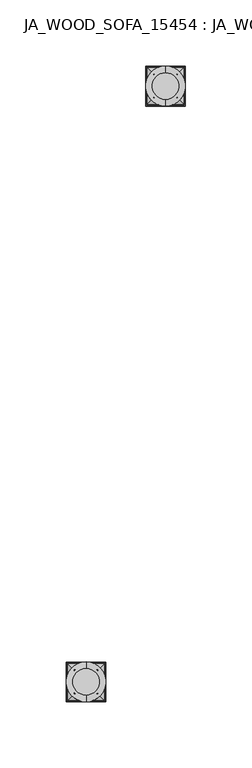
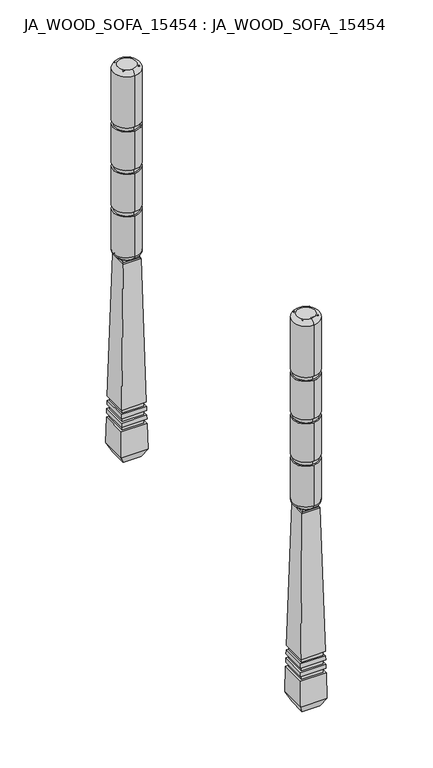
"""IFC4 building model written with IfcOpenShell, lengths in millimetres: furniture geometry, JA_WOOD_SOFA_15454 : JA_WOOD_SOFA_15454."""

from ifc_helpers import new_model, si_unit, point, frame, origin, origin_with_axes, place, context, project, spatial, polyline, circle_curve, ellipse_curve, trimmed, outline, extrude, faceted_brep, source, transform, mapped, element, save
from ifc_brep_helpers import plane_surface, cylinder_surface, revolved_surface, advanced_brep


def ja_wood_sofa_15454_ja_wood_sofa_15454_b7308ffd(model_context):
    return source(origin(), model_context, "Body", "SolidModel", [
        advanced_brep(
        [(-237.5, 460.0, 460.0), (-237.5, 440.0, 460.0), (-237.5, 442.0710678, 235.0), (-237.5, 457.9289322, 235.0), (-237.5, 465.0, 245.0), (-237.5, 465.0, 242.0710678), (-237.5, 435.0, 242.0710678), (-237.5, 435.0, 245.0), (-237.5, 435.0, 290.0), (-237.5, 465.0, 290.0), (-237.5, 465.0, 455.0000045), (-237.5, 465.0, 450.0), (-237.5, 465.0, 395.0), (-237.5, 435.0, 395.0), (-237.5, 435.0, 450.0), (-237.5, 435.0, 455.0000074), (-237.5, 465.0, 390.0), (-237.5, 465.0, 345.0), (-237.5, 435.0, 345.0), (-237.5, 435.0, 390.0), (-237.5, 465.0, 340.0), (-237.5, 465.0, 295.0), (-237.5, 435.0, 295.0), (-237.5, 435.0, 340.0), (-237.5, 436.4644661, 238.5355339), (-237.5, 463.5355339, 238.5355339), (-237.5, 461.4644661, 236.4644661), (-237.5, 438.5355339, 236.4644661), (-237.5, 437.0, 340.0), (-237.5, 437.0, 345.0), (-237.5, 463.0, 345.0), (-237.5, 463.0, 340.0), (-237.5, 437.0, 390.0), (-237.5, 437.0, 395.0), (-237.5, 463.0, 395.0), (-237.5, 463.0, 390.0), (-237.5, 437.0, 290.0), (-237.5, 437.0, 295.0), (-237.5, 463.0, 295.0), (-237.5, 463.0, 290.0)],
        [
            (0, 1, circle_curve(frame((-237.5, 450.0, 460.0), z_axis=(0.0, 0.0, 1.0), x_axis=(0.0, 1.0, 0.0)), 10.0)),
            (1, 0, circle_curve(frame((-237.5, 450.0, 460.0), z_axis=(0.0, 0.0, 1.0), x_axis=(0.0, -1.0, 0.0)), 10.0)),
            (2, 3, circle_curve(frame((-237.5, 450.0, 235.0), z_axis=(0.0, 0.0, -1.0), x_axis=(0.0, 1.0, 0.0)), 7.9289322)),
            (3, 2, circle_curve(frame((-237.5, 450.0, 235.0), z_axis=(0.0, 0.0, -1.0), x_axis=(0.0, -1.0, 0.0)), 7.9289322)),
            (4, 5),
            (5, 6, circle_curve(frame((-237.5, 450.0, 242.0710678), z_axis=(0.0, 0.0, 1.0), x_axis=(0.0, -1.0, 0.0)), 15.0)),
            (6, 7),
            (7, 8),
            (8, 9, circle_curve(frame((-237.5, 450.0, 290.0), z_axis=(0.0, 0.0, -1.0), x_axis=(0.0, -1.0, 0.0)), 15.0)),
            (9, 4),
            (10, 11),
            (11, 12),
            (12, 13, circle_curve(frame((-237.5, 450.0, 395.0), z_axis=(0.0, 0.0, 1.0), x_axis=(0.0, -1.0, 0.0)), 15.0)),
            (13, 14),
            (14, 15),
            (15, 10, circle_curve(frame((-237.5, 450.0, 455.0), z_axis=(0.0, 0.0, -1.0), x_axis=(0.0, -1.0, 0.0)), 15.0)),
            (16, 17),
            (17, 18, circle_curve(frame((-237.5, 450.0, 345.0), z_axis=(0.0, 0.0, 1.0), x_axis=(0.0, -1.0, 0.0)), 15.0)),
            (18, 19),
            (19, 16, circle_curve(frame((-237.5, 450.0, 390.0), z_axis=(0.0, 0.0, -1.0), x_axis=(0.0, -1.0, 0.0)), 15.0)),
            (20, 21),
            (21, 22, circle_curve(frame((-237.5, 450.0, 295.0), z_axis=(0.0, 0.0, 1.0), x_axis=(0.0, -1.0, 0.0)), 15.0)),
            (22, 23),
            (23, 20, circle_curve(frame((-237.5, 450.0, 340.0), z_axis=(0.0, 0.0, -1.0), x_axis=(0.0, -1.0, 0.0)), 15.0)),
            (9, 8, circle_curve(frame((-237.5, 450.0, 290.0), z_axis=(0.0, 0.0, -1.0), x_axis=(0.0, -1.0, 0.0)), 15.0)),
            (6, 5, circle_curve(frame((-237.5, 450.0, 242.0710678), z_axis=(0.0, 0.0, 1.0), x_axis=(0.0, -1.0, 0.0)), 15.0)),
            (10, 15, circle_curve(frame((-237.5, 450.0, 455.0), z_axis=(0.0, 0.0, -1.0), x_axis=(0.0, -1.0, 0.0)), 15.0)),
            (13, 12, circle_curve(frame((-237.5, 450.0, 395.0), z_axis=(0.0, 0.0, 1.0), x_axis=(0.0, -1.0, 0.0)), 15.0)),
            (16, 19, circle_curve(frame((-237.5, 450.0, 390.0), z_axis=(0.0, 0.0, -1.0), x_axis=(0.0, -1.0, 0.0)), 15.0)),
            (18, 17, circle_curve(frame((-237.5, 450.0, 345.0), z_axis=(0.0, 0.0, 1.0), x_axis=(0.0, -1.0, 0.0)), 15.0)),
            (20, 23, circle_curve(frame((-237.5, 450.0, 340.0), z_axis=(0.0, 0.0, -1.0), x_axis=(0.0, -1.0, 0.0)), 15.0)),
            (22, 21, circle_curve(frame((-237.5, 450.0, 295.0), z_axis=(0.0, 0.0, 1.0), x_axis=(0.0, -1.0, 0.0)), 15.0)),
            (24, 6, circle_curve(frame((-237.5, 440.0, 242.0710678), z_axis=(-1.0, 0.0, 0.0), x_axis=(0.0, -1.0, 0.0)), 5.0)),
            (5, 25, circle_curve(frame((-237.5, 460.0, 242.0710678), z_axis=(-1.0, 0.0, 0.0), x_axis=(0.0, 1.0, 0.0)), 5.0)),
            (25, 24, circle_curve(frame((-237.5, 450.0, 238.5355339), z_axis=(0.0, 0.0, 1.0), x_axis=(0.0, 1.0, 0.0)), 13.5355339)),
            (25, 26),
            (26, 27, circle_curve(frame((-237.5, 450.0, 236.4644661), z_axis=(0.0, 0.0, 1.0), x_axis=(0.0, 1.0, 0.0)), 11.4644661)),
            (27, 24),
            (26, 3, circle_curve(frame((-237.5, 457.9289322, 240.0), z_axis=(-1.0, 0.0, 0.0), x_axis=(0.0, 1.0, 0.0)), 5.0)),
            (2, 27, circle_curve(frame((-237.5, 442.0710678, 240.0), z_axis=(-1.0, 0.0, 0.0), x_axis=(0.0, -1.0, 0.0)), 5.0)),
            (24, 25, circle_curve(frame((-237.5, 450.0, 238.5355339), z_axis=(0.0, 0.0, 1.0), x_axis=(0.0, -1.0, 0.0)), 13.5355339)),
            (27, 26, circle_curve(frame((-237.5, 450.0, 236.4644661), z_axis=(0.0, 0.0, 1.0), x_axis=(0.0, -1.0, 0.0)), 11.4644661)),
            (15, 1, circle_curve(frame((-237.5, 440.0, 455.0), z_axis=(-1.0, 0.0, 0.0), x_axis=(0.0, -1.0, 0.0)), 5.0)),
            (0, 10, circle_curve(frame((-237.5, 460.0, 455.0), z_axis=(-1.0, 0.0, 0.0), x_axis=(0.0, 1.0, 0.0)), 5.0)),
            (28, 29),
            (29, 30, circle_curve(frame((-237.5, 450.0, 345.0), z_axis=(0.0, 0.0, -1.0), x_axis=(0.0, 1.0, 0.0)), 13.0)),
            (30, 31),
            (31, 28, circle_curve(frame((-237.5, 450.0, 340.0), z_axis=(0.0, 0.0, 1.0), x_axis=(0.0, 1.0, 0.0)), 13.0)),
            (32, 33),
            (33, 34, circle_curve(frame((-237.5, 450.0, 395.0), z_axis=(0.0, 0.0, -1.0), x_axis=(0.0, 1.0, 0.0)), 13.0)),
            (34, 35),
            (35, 32, circle_curve(frame((-237.5, 450.0, 390.0), z_axis=(0.0, 0.0, 1.0), x_axis=(0.0, 1.0, 0.0)), 13.0)),
            (36, 37),
            (37, 38, circle_curve(frame((-237.5, 450.0, 295.0), z_axis=(0.0, 0.0, -1.0), x_axis=(0.0, 1.0, 0.0)), 13.0)),
            (38, 39),
            (39, 36, circle_curve(frame((-237.5, 450.0, 290.0), z_axis=(0.0, 0.0, 1.0), x_axis=(0.0, 1.0, 0.0)), 13.0)),
            (28, 31, circle_curve(frame((-237.5, 450.0, 340.0), z_axis=(0.0, 0.0, 1.0), x_axis=(0.0, -1.0, 0.0)), 13.0)),
            (30, 29, circle_curve(frame((-237.5, 450.0, 345.0), z_axis=(0.0, 0.0, -1.0), x_axis=(0.0, -1.0, 0.0)), 13.0)),
            (32, 35, circle_curve(frame((-237.5, 450.0, 390.0), z_axis=(0.0, 0.0, 1.0), x_axis=(0.0, -1.0, 0.0)), 13.0)),
            (34, 33, circle_curve(frame((-237.5, 450.0, 395.0), z_axis=(0.0, 0.0, -1.0), x_axis=(0.0, -1.0, 0.0)), 13.0)),
            (36, 39, circle_curve(frame((-237.5, 450.0, 290.0), z_axis=(0.0, 0.0, 1.0), x_axis=(0.0, -1.0, 0.0)), 13.0)),
            (38, 37, circle_curve(frame((-237.5, 450.0, 295.0), z_axis=(0.0, 0.0, -1.0), x_axis=(0.0, -1.0, 0.0)), 13.0)),
        ],
        [
            plane_surface(frame((-237.5, 435.0, 460.0), z_axis=(0.0, 0.0, 1.0), x_axis=(1.0, 0.0, 0.0))),
            plane_surface(frame((-237.5, 435.0, 235.0), z_axis=(0.0, 0.0, -1.0), x_axis=(-1.0, 0.0, 0.0))),
            cylinder_surface(frame((-237.5, 450.0, 235.0), z_axis=(0.0, 0.0, 1.0), x_axis=(0.0, -1.0, 0.0)), 15.0),
            revolved_surface(trimmed(ellipse_curve(frame((-237.5, 460.0, 242.0710678), z_axis=(1.0, 0.0, 0.0), x_axis=(0.0, 1.0, 0.0)), 5.0, 5.0), [point((-237.5, 463.5355339, 238.5355339))], [point((-237.5, 465.0, 242.0710678))], True, "CARTESIAN"), (-237.5, 450.0, 235.0), (0.0, 0.0, 1.0)),
            revolved_surface(polyline([(-237.5, 461.4644661, 236.4644661), (-237.5, 463.5355339, 238.5355339)]), (-237.5, 450.0, 235.0), (0.0, 0.0, 1.0)),
            revolved_surface(trimmed(ellipse_curve(frame((-237.5, 457.9289322, 240.0), z_axis=(1.0, 0.0, 0.0), x_axis=(0.0, 1.0, 0.0)), 5.0, 5.0), [point((-237.5, 457.9289322, 235.0))], [point((-237.5, 461.4644661, 236.4644661))], True, "CARTESIAN"), (-237.5, 450.0, 235.0), (0.0, 0.0, 1.0)),
            revolved_surface(trimmed(ellipse_curve(frame((-237.5, 440.0, 242.0710678), z_axis=(-1.0, 0.0, 0.0), x_axis=(0.0, -1.0, 0.0)), 5.0, 5.0), [point((-237.5, 436.4644661, 238.5355339))], [point((-237.5, 435.0, 242.0710678))], True, "CARTESIAN"), (-237.5, 450.0, 235.0), (0.0, 0.0, 1.0)),
            revolved_surface(polyline([(-237.5, 438.5355339, 236.4644661), (-237.5, 436.4644661, 238.5355339)]), (-237.5, 450.0, 235.0), (0.0, 0.0, 1.0)),
            revolved_surface(trimmed(ellipse_curve(frame((-237.5, 442.0710678, 240.0), z_axis=(-1.0, 0.0, 0.0), x_axis=(0.0, -1.0, 0.0)), 5.0, 5.0), [point((-237.5, 442.0710678, 235.0))], [point((-237.5, 438.5355339, 236.4644661))], True, "CARTESIAN"), (-237.5, 450.0, 235.0), (0.0, 0.0, 1.0)),
            revolved_surface(trimmed(ellipse_curve(frame((-237.5, 460.0, 455.0), z_axis=(1.0, 0.0, 0.0), x_axis=(0.0, 1.0, 0.0)), 5.0, 5.0), [point((-237.5, 465.0, 455.0))], [point((-237.5, 460.0, 460.0))], True, "CARTESIAN"), (-237.5, 450.0, 235.0), (0.0, 0.0, 1.0)),
            revolved_surface(trimmed(ellipse_curve(frame((-237.5, 440.0, 455.0), z_axis=(-1.0, 0.0, 0.0), x_axis=(0.0, -1.0, 0.0)), 5.0, 5.0), [point((-237.5, 435.0, 455.0))], [point((-237.5, 440.0, 460.0))], True, "CARTESIAN"), (-237.5, 450.0, 235.0), (0.0, 0.0, 1.0)),
            cylinder_surface(frame((-237.5, 450.0, 235.0), z_axis=(0.0, 0.0, 1.0), x_axis=(0.0, 1.0, 0.0)), 13.0),
            cylinder_surface(frame((-237.5, 450.0, 235.0), z_axis=(0.0, 0.0, 1.0), x_axis=(0.0, -1.0, 0.0)), 13.0),
            plane_surface(frame((-237.5, 450.0, 340.0), z_axis=(0.0, 0.0, 1.0), x_axis=(0.0, -1.0, 0.0))),
            plane_surface(frame((-237.5, 450.0, 345.0), z_axis=(0.0, 0.0, -1.0), x_axis=(0.0, -1.0, 0.0))),
            plane_surface(frame((-237.5, 450.0, 390.0), z_axis=(0.0, 0.0, 1.0), x_axis=(0.0, -1.0, 0.0))),
            plane_surface(frame((-237.5, 450.0, 395.0), z_axis=(0.0, 0.0, -1.0), x_axis=(0.0, -1.0, 0.0))),
            plane_surface(frame((-237.5, 450.0, 290.0), z_axis=(0.0, 0.0, 1.0), x_axis=(0.0, -1.0, 0.0))),
            plane_surface(frame((-237.5, 450.0, 295.0), z_axis=(0.0, 0.0, -1.0), x_axis=(0.0, -1.0, 0.0))),
        ],
        [
            (0, [[1, 2]]),
            (1, [[3, 4]]),
            (2, [[5, 6, 7, 8, 9, 10]]),
            (2, [[11, 12, 13, 14, 15, 16]]),
            (2, [[17, 18, 19, 20]]),
            (2, [[21, 22, 23, 24]]),
            (2, [[-5, -10, 25, -8, -7, 26]]),
            (2, [[-11, 27, -15, -14, 28, -12]]),
            (2, [[-17, 29, -19, 30]]),
            (2, [[-21, 31, -23, 32]]),
            (3, [[33, -6, 34, 35]]),
            (4, [[-35, 36, 37, 38]]),
            (5, [[-37, 39, -3, 40]]),
            (6, [[-33, 41, -34, -26]]),
            (7, [[-38, 42, -36, -41]]),
            (8, [[-40, -4, -39, -42]]),
            (9, [[43, -1, 44, -16]]),
            (10, [[-43, -27, -44, -2]]),
            (11, [[45, 46, 47, 48]]),
            (11, [[49, 50, 51, 52]]),
            (11, [[53, 54, 55, 56]]),
            (12, [[-45, 57, -47, 58]]),
            (13, [[-24, -31], [-48, -57]]),
            (14, [[-18, -30], [-46, -58]]),
            (12, [[-49, 59, -51, 60]]),
            (15, [[-20, -29], [-52, -59]]),
            (16, [[-13, -28], [-50, -60]]),
            (12, [[-53, 61, -55, 62]]),
            (17, [[-9, -25], [-56, -61]]),
            (18, [[-22, -32], [-54, -62]]),
        ],
    ),
        extrude(outline(polyline([(-228.5, 459.0), (-228.5, 441.0), (-246.5, 441.0), (-246.5, 459.0), (-228.5, 459.0)])), origin_with_axes(), (0.0, 0.0, 1.0), 460.0),
        advanced_brep(
        [(-251.2777778, 463.7777778, 65.0), (-247.543457, 460.043457, 233.0444335), (-227.456543, 460.043457, 233.0444335), (-223.7222222, 463.7777778, 65.0), (-227.456543, 439.956543, 233.0444335), (-223.7222222, 436.2222222, 65.0), (-247.543457, 439.956543, 233.0444335), (-251.2777778, 436.2222222, 65.0), (-222.5, 465.0, 10.0), (-222.5, 435.0, 10.0), (-252.5, 435.0, 10.0), (-252.5, 465.0, 10.0), (-242.5, 455.0, 10.0), (-242.5, 445.0, 10.0), (-232.5, 445.0, 10.0), (-232.5, 455.0, 10.0), (-249.5, 462.0, 60.0), (-249.5, 462.0, 65.0), (-225.5, 462.0, 65.0), (-225.5, 462.0, 60.0), (-251.5, 464.0, 55.0), (-251.3888889, 463.8888889, 60.0), (-223.6111111, 463.8888889, 60.0), (-223.5, 464.0, 55.0), (-249.5, 462.0, 50.0), (-249.5, 462.0, 55.0), (-225.5, 462.0, 55.0), (-225.5, 462.0, 50.0), (-251.7222222, 464.2222222, 45.0), (-251.6111111, 464.1111111, 50.0), (-223.3888889, 464.1111111, 50.0), (-223.2777778, 464.2222222, 45.0), (-249.5, 462.0, 40.0), (-249.5, 462.0, 45.0), (-225.5, 462.0, 45.0), (-225.5, 462.0, 40.0), (-251.8333333, 464.3333333, 40.0), (-223.1666667, 464.3333333, 40.0), (-225.5, 438.0, 65.0), (-225.5, 438.0, 60.0), (-223.6111111, 436.1111111, 60.0), (-223.5, 436.0, 55.0), (-225.5, 438.0, 55.0), (-225.5, 438.0, 50.0), (-223.3888889, 435.8888889, 50.0), (-223.2777778, 435.7777778, 45.0), (-225.5, 438.0, 45.0), (-225.5, 438.0, 40.0), (-223.1666667, 435.6666667, 40.0), (-249.5, 438.0, 65.0), (-249.5, 438.0, 60.0), (-251.3888889, 436.1111111, 60.0), (-251.5, 436.0, 55.0), (-249.5, 438.0, 55.0), (-249.5, 438.0, 50.0), (-251.6111111, 435.8888889, 50.0), (-251.7222222, 435.7777778, 45.0), (-249.5, 438.0, 45.0), (-249.5, 438.0, 40.0), (-251.8333333, 435.6666667, 40.0), (-242.5, 455.0, 235.0), (-232.5, 455.0, 235.0), (-245.5439507, 458.0439507, 235.0), (-229.4560493, 458.0439507, 235.0), (-232.5, 445.0, 235.0), (-229.4560493, 441.9560493, 235.0), (-242.5, 445.0, 235.0), (-245.5439507, 441.9560493, 235.0)],
        [
            (0, 1),
            (1, 2),
            (2, 3),
            (3, 0),
            (2, 4),
            (4, 5),
            (5, 3),
            (4, 6),
            (6, 7),
            (7, 5),
            (6, 1),
            (0, 7),
            (8, 9),
            (9, 10),
            (10, 11),
            (11, 8),
            (12, 13),
            (13, 14),
            (14, 15),
            (15, 12),
            (16, 17),
            (17, 18),
            (18, 19),
            (19, 16),
            (20, 21),
            (21, 22),
            (22, 23),
            (23, 20),
            (24, 25),
            (25, 26),
            (26, 27),
            (27, 24),
            (28, 29),
            (29, 30),
            (30, 31),
            (31, 28),
            (32, 33),
            (33, 34),
            (34, 35),
            (35, 32),
            (11, 36),
            (36, 37),
            (37, 8),
            (18, 38),
            (38, 39),
            (39, 19),
            (22, 40),
            (40, 41),
            (41, 23),
            (26, 42),
            (42, 43),
            (43, 27),
            (30, 44),
            (44, 45),
            (45, 31),
            (34, 46),
            (46, 47),
            (47, 35),
            (37, 48),
            (48, 9),
            (38, 49),
            (49, 50),
            (50, 39),
            (40, 51),
            (51, 52),
            (52, 41),
            (42, 53),
            (53, 54),
            (54, 43),
            (44, 55),
            (55, 56),
            (56, 45),
            (46, 57),
            (57, 58),
            (58, 47),
            (48, 59),
            (59, 10),
            (17, 49),
            (16, 50),
            (21, 51),
            (20, 52),
            (25, 53),
            (24, 54),
            (29, 55),
            (28, 56),
            (33, 57),
            (32, 58),
            (36, 59),
            (60, 12),
            (15, 61),
            (61, 60),
            (1, 62, ellipse_curve(frame((-245.5439507, 458.0439507, 233.0), z_axis=(0.7071067811865471, 0.7071067811865477, 0.0), x_axis=(-0.707106781186548, 0.707106781186547, 0.0)), 2.8284271, 2.0)),
            (62, 63),
            (63, 2, ellipse_curve(frame((-229.4560493, 458.0439507, 233.0), z_axis=(-0.7071067811865476, 0.7071067811865474, 0.0), x_axis=(-0.7071067811865476, -0.7071067811865475, 0.0)), 2.8284271, 2.0)),
            (14, 64),
            (64, 61),
            (63, 65),
            (65, 4, ellipse_curve(frame((-229.4560493, 441.9560493, 233.0), z_axis=(0.7071067811865475, 0.7071067811865476, 0.0), x_axis=(-0.7071067811865475, 0.7071067811865475, 0.0)), 2.8284271, 2.0)),
            (13, 66),
            (66, 64),
            (65, 67),
            (67, 6, ellipse_curve(frame((-245.5439507, 441.9560493, 233.0), z_axis=(0.7071067811865477, -0.7071067811865472, 0.0), x_axis=(0.7071067811865474, 0.7071067811865476, 0.0)), 2.8284271, 2.0)),
            (60, 66),
            (62, 67),
        ],
        [
            plane_surface(frame((-247.543457, 460.043457, 233.0444335), z_axis=(0.0, 0.99975317783161, 0.022216737285146875), x_axis=(1.0, 0.0, 0.0))),
            plane_surface(frame((-227.456543, 460.043457, 233.0444335), z_axis=(0.99975317783161, 0.0, 0.022216737285146875), x_axis=(0.0, -1.0, 0.0))),
            plane_surface(frame((-227.456543, 439.956543, 233.0444335), z_axis=(0.0, -0.99975317783161, 0.02221673728514687), x_axis=(-1.0, 0.0, 0.0))),
            plane_surface(frame((-247.543457, 439.956543, 233.0444335), z_axis=(-0.99975317783161, 0.0, 0.022216737285146868), x_axis=(0.0, 1.0, 0.0))),
            plane_surface(frame((-252.5, 435.0, 10.0), z_axis=(0.0, 0.0, -1.0), x_axis=(0.0, 1.0, 0.0))),
            plane_surface(frame((-249.5, 462.0, 65.0), z_axis=(0.0, 1.0, 0.0), x_axis=(1.0, 0.0, 0.0))),
            plane_surface(frame((-251.3888889, 463.8888889, 60.0), z_axis=(0.0, 0.99975317783161, 0.022216737285146875), x_axis=(1.0, 0.0, 0.0))),
            plane_surface(frame((-249.5, 462.0, 55.0), z_axis=(0.0, 1.0, 0.0), x_axis=(1.0, 0.0, 0.0))),
            plane_surface(frame((-251.6111111, 464.1111111, 50.0), z_axis=(0.0, 0.99975317783161, 0.022216737285146875), x_axis=(1.0, 0.0, 0.0))),
            plane_surface(frame((-249.5, 462.0, 45.0), z_axis=(0.0, 1.0, 0.0), x_axis=(1.0, 0.0, 0.0))),
            plane_surface(frame((-251.8333333, 464.3333333, 40.0), z_axis=(0.0, 0.99975317783161, 0.022216737285146875), x_axis=(1.0, 0.0, 0.0))),
            plane_surface(frame((-225.5, 462.0, 65.0), z_axis=(1.0, 0.0, 0.0), x_axis=(0.0, -1.0, 0.0))),
            plane_surface(frame((-223.6111111, 463.8888889, 60.0), z_axis=(0.99975317783161, 0.0, 0.022216737285146875), x_axis=(0.0, -1.0, 0.0))),
            plane_surface(frame((-225.5, 462.0, 55.0), z_axis=(1.0, 0.0, 0.0), x_axis=(0.0, -1.0, 0.0))),
            plane_surface(frame((-223.3888889, 464.1111111, 50.0), z_axis=(0.99975317783161, 0.0, 0.022216737285146875), x_axis=(0.0, -1.0, 0.0))),
            plane_surface(frame((-225.5, 462.0, 45.0), z_axis=(1.0, 0.0, 0.0), x_axis=(0.0, -1.0, 0.0))),
            plane_surface(frame((-223.1666667, 464.3333333, 40.0), z_axis=(0.99975317783161, 0.0, 0.022216737285146875), x_axis=(0.0, -1.0, 0.0))),
            plane_surface(frame((-225.5, 438.0, 65.0), z_axis=(0.0, -1.0, 0.0), x_axis=(-1.0, 0.0, 0.0))),
            plane_surface(frame((-223.6111111, 436.1111111, 60.0), z_axis=(0.0, -0.99975317783161, 0.02221673728514687), x_axis=(-1.0, 0.0, 0.0))),
            plane_surface(frame((-225.5, 438.0, 55.0), z_axis=(0.0, -1.0, 0.0), x_axis=(-1.0, 0.0, 0.0))),
            plane_surface(frame((-223.3888889, 435.8888889, 50.0), z_axis=(0.0, -0.99975317783161, 0.02221673728514687), x_axis=(-1.0, 0.0, 0.0))),
            plane_surface(frame((-225.5, 438.0, 45.0), z_axis=(0.0, -1.0, 0.0), x_axis=(-1.0, 0.0, 0.0))),
            plane_surface(frame((-223.1666667, 435.6666667, 40.0), z_axis=(0.0, -0.99975317783161, 0.02221673728514687), x_axis=(-1.0, 0.0, 0.0))),
            plane_surface(frame((-251.2777778, 436.2222222, 65.0), z_axis=(0.0, 0.0, -1.0), x_axis=(0.0, 1.0, 0.0))),
            plane_surface(frame((-249.5, 438.0, 65.0), z_axis=(-1.0, 0.0, 0.0), x_axis=(0.0, 1.0, 0.0))),
            plane_surface(frame((-249.5, 438.0, 60.0), z_axis=(0.0, 0.0, 1.0), x_axis=(0.0, 1.0, 0.0))),
            plane_surface(frame((-251.3888889, 436.1111111, 60.0), z_axis=(-0.99975317783161, 0.0, 0.022216737285146868), x_axis=(0.0, 1.0, 0.0))),
            plane_surface(frame((-251.5, 436.0, 55.0), z_axis=(0.0, 0.0, -1.0), x_axis=(0.0, 1.0, 0.0))),
            plane_surface(frame((-249.5, 438.0, 55.0), z_axis=(-1.0, 0.0, 0.0), x_axis=(0.0, 1.0, 0.0))),
            plane_surface(frame((-249.5, 438.0, 50.0), z_axis=(0.0, 0.0, 1.0), x_axis=(0.0, 1.0, 0.0))),
            plane_surface(frame((-251.6111111, 435.8888889, 50.0), z_axis=(-0.99975317783161, 0.0, 0.022216737285146868), x_axis=(0.0, 1.0, 0.0))),
            plane_surface(frame((-251.7222222, 435.7777778, 45.0), z_axis=(0.0, 0.0, -1.0), x_axis=(0.0, 1.0, 0.0))),
            plane_surface(frame((-249.5, 438.0, 45.0), z_axis=(-1.0, 0.0, 0.0), x_axis=(0.0, 1.0, 0.0))),
            plane_surface(frame((-249.5, 438.0, 40.0), z_axis=(0.0, 0.0, 1.0), x_axis=(0.0, 1.0, 0.0))),
            plane_surface(frame((-251.8333333, 435.6666667, 40.0), z_axis=(-0.99975317783161, 0.0, 0.022216737285146868), x_axis=(0.0, 1.0, 0.0))),
            plane_surface(frame((-242.5, 455.0, 10.0), z_axis=(0.0, -1.0, 0.0), x_axis=(1.0, 0.0, 0.0))),
            cylinder_surface(frame((-252.5, 458.0439507, 233.0), z_axis=(-1.0, 0.0, 0.0), x_axis=(0.0, 1.0, 0.0)), 2.0),
            plane_surface(frame((-232.5, 455.0, 10.0), z_axis=(-1.0, 0.0, 0.0), x_axis=(0.0, -1.0, 0.0))),
            cylinder_surface(frame((-229.4560493, 465.0, 233.0), z_axis=(0.0, 1.0, 0.0), x_axis=(1.0, 0.0, 0.0)), 2.0),
            plane_surface(frame((-232.5, 445.0, 10.0), z_axis=(0.0, 1.0, 0.0), x_axis=(-1.0, 0.0, 0.0))),
            cylinder_surface(frame((-222.5, 441.9560493, 233.0), z_axis=(1.0, 0.0, 0.0), x_axis=(0.0, -1.0, 0.0)), 2.0),
            plane_surface(frame((-242.5, 445.0, 10.0), z_axis=(1.0, 0.0, 0.0), x_axis=(0.0, 1.0, 0.0))),
            plane_surface(frame((-242.5, 445.0, 235.0), z_axis=(0.0, 0.0, 1.0), x_axis=(0.0, 1.0, 0.0))),
            cylinder_surface(frame((-245.5439507, 435.0, 233.0), z_axis=(0.0, -1.0, 0.0), x_axis=(-1.0, 0.0, 0.0)), 2.0),
        ],
        [
            (0, [[1, 2, 3, 4]]),
            (1, [[-3, 5, 6, 7]]),
            (2, [[-6, 8, 9, 10]]),
            (3, [[-9, 11, -1, 12]]),
            (4, [[13, 14, 15, 16], [17, 18, 19, 20]]),
            (5, [[21, 22, 23, 24]]),
            (6, [[25, 26, 27, 28]]),
            (7, [[29, 30, 31, 32]]),
            (8, [[33, 34, 35, 36]]),
            (9, [[37, 38, 39, 40]]),
            (10, [[41, 42, 43, -16]]),
            (11, [[-23, 44, 45, 46]]),
            (12, [[-27, 47, 48, 49]]),
            (13, [[-31, 50, 51, 52]]),
            (14, [[-35, 53, 54, 55]]),
            (15, [[-39, 56, 57, 58]]),
            (16, [[-43, 59, 60, -13]]),
            (17, [[-45, 61, 62, 63]]),
            (18, [[-48, 64, 65, 66]]),
            (19, [[-51, 67, 68, 69]]),
            (20, [[-54, 70, 71, 72]]),
            (21, [[-57, 73, 74, 75]]),
            (22, [[-60, 76, 77, -14]]),
            (23, [[-7, -10, -12, -4], [78, -61, -44, -22]]),
            (24, [[-62, -78, -21, 79]]),
            (25, [[80, -64, -47, -26], [-46, -63, -79, -24]]),
            (26, [[-65, -80, -25, 81]]),
            (27, [[-49, -66, -81, -28], [82, -67, -50, -30]]),
            (28, [[-68, -82, -29, 83]]),
            (29, [[84, -70, -53, -34], [-52, -69, -83, -32]]),
            (30, [[-71, -84, -33, 85]]),
            (31, [[-55, -72, -85, -36], [86, -73, -56, -38]]),
            (32, [[-74, -86, -37, 87]]),
            (33, [[88, -76, -59, -42], [-58, -75, -87, -40]]),
            (34, [[-77, -88, -41, -15]]),
            (35, [[89, -20, 90, 91]]),
            (36, [[92, 93, 94, -2]]),
            (37, [[-90, -19, 95, 96]]),
            (38, [[-94, 97, 98, -5]]),
            (39, [[-95, -18, 99, 100]]),
            (40, [[-98, 101, 102, -8]]),
            (41, [[-99, -17, -89, 103]]),
            (42, [[104, -101, -97, -93], [-96, -100, -103, -91]]),
            (43, [[-102, -104, -92, -11]]),
        ],
    ),
        faceted_brep([(-222.5, 435.0, 10.0), (-222.5, 465.0, 10.0), (-252.5, 465.0, 10.0), (-252.5, 435.0, 10.0), (-227.5, 440.0, 0.0), (-247.5, 440.0, 0.0), (-247.5, 460.0, 0.0), (-227.5, 460.0, 0.0)], [[[0, 1, 2, 3]], [[4, 5, 6, 7]], [[4, 7, 1, 0]], [[7, 6, 2, 1]], [[6, 5, 3, 2]], [[5, 4, 0, 3]]]),
        advanced_brep(
        [(-297.5, 10.0, 460.0), (-297.5, -10.0, 460.0), (-297.5, -7.9289322, 235.0), (-297.5, 7.9289322, 235.0), (-297.5, 15.0, 245.0), (-297.5, 15.0, 242.0710678), (-297.5, -15.0, 242.0710678), (-297.5, -15.0, 245.0), (-297.5, -15.0, 290.0), (-297.5, 15.0, 290.0), (-297.5, 15.0, 455.0000045), (-297.5, 15.0, 450.0), (-297.5, 15.0, 395.0), (-297.5, -15.0, 395.0), (-297.5, -15.0, 450.0), (-297.5, -15.0, 455.0000074), (-297.5, 15.0, 390.0), (-297.5, 15.0, 345.0), (-297.5, -15.0, 345.0), (-297.5, -15.0, 390.0), (-297.5, 15.0, 340.0), (-297.5, 15.0, 295.0), (-297.5, -15.0, 295.0), (-297.5, -15.0, 340.0), (-297.5, -13.5355339, 238.5355339), (-297.5, 13.5355339, 238.5355339), (-297.5, 11.4644661, 236.4644661), (-297.5, -11.4644661, 236.4644661), (-297.5, -13.0, 340.0), (-297.5, -13.0, 345.0), (-297.5, 13.0, 345.0), (-297.5, 13.0, 340.0), (-297.5, -13.0, 390.0), (-297.5, -13.0, 395.0), (-297.5, 13.0, 395.0), (-297.5, 13.0, 390.0), (-297.5, -13.0, 290.0), (-297.5, -13.0, 295.0), (-297.5, 13.0, 295.0), (-297.5, 13.0, 290.0)],
        [
            (0, 1, circle_curve(frame((-297.5, 0.0, 460.0), z_axis=(0.0, 0.0, 1.0), x_axis=(0.0, 1.0, 0.0)), 10.0)),
            (1, 0, circle_curve(frame((-297.5, 0.0, 460.0), z_axis=(0.0, 0.0, 1.0), x_axis=(0.0, -1.0, 0.0)), 10.0)),
            (2, 3, circle_curve(frame((-297.5, 0.0, 235.0), z_axis=(0.0, 0.0, -1.0), x_axis=(0.0, 1.0, 0.0)), 7.9289322)),
            (3, 2, circle_curve(frame((-297.5, 0.0, 235.0), z_axis=(0.0, 0.0, -1.0), x_axis=(0.0, -1.0, 0.0)), 7.9289322)),
            (4, 5),
            (5, 6, circle_curve(frame((-297.5, 0.0, 242.0710678), z_axis=(0.0, 0.0, 1.0), x_axis=(0.0, -1.0, 0.0)), 15.0)),
            (6, 7),
            (7, 8),
            (8, 9, circle_curve(frame((-297.5, 0.0, 290.0), z_axis=(0.0, 0.0, -1.0), x_axis=(0.0, -1.0, 0.0)), 15.0)),
            (9, 4),
            (10, 11),
            (11, 12),
            (12, 13, circle_curve(frame((-297.5, 0.0, 395.0), z_axis=(0.0, 0.0, 1.0), x_axis=(0.0, -1.0, 0.0)), 15.0)),
            (13, 14),
            (14, 15),
            (15, 10, circle_curve(frame((-297.5, 0.0, 455.0), z_axis=(0.0, 0.0, -1.0), x_axis=(0.0, -1.0, 0.0)), 15.0)),
            (16, 17),
            (17, 18, circle_curve(frame((-297.5, 0.0, 345.0), z_axis=(0.0, 0.0, 1.0), x_axis=(0.0, -1.0, 0.0)), 15.0)),
            (18, 19),
            (19, 16, circle_curve(frame((-297.5, 0.0, 390.0), z_axis=(0.0, 0.0, -1.0), x_axis=(0.0, -1.0, 0.0)), 15.0)),
            (20, 21),
            (21, 22, circle_curve(frame((-297.5, 0.0, 295.0), z_axis=(0.0, 0.0, 1.0), x_axis=(0.0, -1.0, 0.0)), 15.0)),
            (22, 23),
            (23, 20, circle_curve(frame((-297.5, 0.0, 340.0), z_axis=(0.0, 0.0, -1.0), x_axis=(0.0, -1.0, 0.0)), 15.0)),
            (9, 8, circle_curve(frame((-297.5, 0.0, 290.0), z_axis=(0.0, 0.0, -1.0), x_axis=(0.0, -1.0, 0.0)), 15.0)),
            (6, 5, circle_curve(frame((-297.5, 0.0, 242.0710678), z_axis=(0.0, 0.0, 1.0), x_axis=(0.0, -1.0, 0.0)), 15.0)),
            (10, 15, circle_curve(frame((-297.5, 0.0, 455.0), z_axis=(0.0, 0.0, -1.0), x_axis=(0.0, -1.0, 0.0)), 15.0)),
            (13, 12, circle_curve(frame((-297.5, 0.0, 395.0), z_axis=(0.0, 0.0, 1.0), x_axis=(0.0, -1.0, 0.0)), 15.0)),
            (16, 19, circle_curve(frame((-297.5, 0.0, 390.0), z_axis=(0.0, 0.0, -1.0), x_axis=(0.0, -1.0, 0.0)), 15.0)),
            (18, 17, circle_curve(frame((-297.5, 0.0, 345.0), z_axis=(0.0, 0.0, 1.0), x_axis=(0.0, -1.0, 0.0)), 15.0)),
            (20, 23, circle_curve(frame((-297.5, 0.0, 340.0), z_axis=(0.0, 0.0, -1.0), x_axis=(0.0, -1.0, 0.0)), 15.0)),
            (22, 21, circle_curve(frame((-297.5, 0.0, 295.0), z_axis=(0.0, 0.0, 1.0), x_axis=(0.0, -1.0, 0.0)), 15.0)),
            (24, 6, circle_curve(frame((-297.5, -10.0, 242.0710678), z_axis=(-1.0, 0.0, 0.0), x_axis=(0.0, -1.0, 0.0)), 5.0)),
            (5, 25, circle_curve(frame((-297.5, 10.0, 242.0710678), z_axis=(-1.0, 0.0, 0.0), x_axis=(0.0, 1.0, 0.0)), 5.0)),
            (25, 24, circle_curve(frame((-297.5, 0.0, 238.5355339), z_axis=(0.0, 0.0, 1.0), x_axis=(0.0, 1.0, 0.0)), 13.5355339)),
            (25, 26),
            (26, 27, circle_curve(frame((-297.5, 0.0, 236.4644661), z_axis=(0.0, 0.0, 1.0), x_axis=(0.0, 1.0, 0.0)), 11.4644661)),
            (27, 24),
            (26, 3, circle_curve(frame((-297.5, 7.9289322, 240.0), z_axis=(-1.0, 0.0, 0.0), x_axis=(0.0, 1.0, 0.0)), 5.0)),
            (2, 27, circle_curve(frame((-297.5, -7.9289322, 240.0), z_axis=(-1.0, 0.0, 0.0), x_axis=(0.0, -1.0, 0.0)), 5.0)),
            (24, 25, circle_curve(frame((-297.5, 0.0, 238.5355339), z_axis=(0.0, 0.0, 1.0), x_axis=(0.0, -1.0, 0.0)), 13.5355339)),
            (27, 26, circle_curve(frame((-297.5, 0.0, 236.4644661), z_axis=(0.0, 0.0, 1.0), x_axis=(0.0, -1.0, 0.0)), 11.4644661)),
            (15, 1, circle_curve(frame((-297.5, -10.0, 455.0), z_axis=(-1.0, 0.0, 0.0), x_axis=(0.0, -1.0, 0.0)), 5.0)),
            (0, 10, circle_curve(frame((-297.5, 10.0, 455.0), z_axis=(-1.0, 0.0, 0.0), x_axis=(0.0, 1.0, 0.0)), 5.0)),
            (28, 29),
            (29, 30, circle_curve(frame((-297.5, 0.0, 345.0), z_axis=(0.0, 0.0, -1.0), x_axis=(0.0, 1.0, 0.0)), 13.0)),
            (30, 31),
            (31, 28, circle_curve(frame((-297.5, 0.0, 340.0), z_axis=(0.0, 0.0, 1.0), x_axis=(0.0, 1.0, 0.0)), 13.0)),
            (32, 33),
            (33, 34, circle_curve(frame((-297.5, 0.0, 395.0), z_axis=(0.0, 0.0, -1.0), x_axis=(0.0, 1.0, 0.0)), 13.0)),
            (34, 35),
            (35, 32, circle_curve(frame((-297.5, 0.0, 390.0), z_axis=(0.0, 0.0, 1.0), x_axis=(0.0, 1.0, 0.0)), 13.0)),
            (36, 37),
            (37, 38, circle_curve(frame((-297.5, 0.0, 295.0), z_axis=(0.0, 0.0, -1.0), x_axis=(0.0, 1.0, 0.0)), 13.0)),
            (38, 39),
            (39, 36, circle_curve(frame((-297.5, 0.0, 290.0), z_axis=(0.0, 0.0, 1.0), x_axis=(0.0, 1.0, 0.0)), 13.0)),
            (28, 31, circle_curve(frame((-297.5, 0.0, 340.0), z_axis=(0.0, 0.0, 1.0), x_axis=(0.0, -1.0, 0.0)), 13.0)),
            (30, 29, circle_curve(frame((-297.5, 0.0, 345.0), z_axis=(0.0, 0.0, -1.0), x_axis=(0.0, -1.0, 0.0)), 13.0)),
            (32, 35, circle_curve(frame((-297.5, 0.0, 390.0), z_axis=(0.0, 0.0, 1.0), x_axis=(0.0, -1.0, 0.0)), 13.0)),
            (34, 33, circle_curve(frame((-297.5, 0.0, 395.0), z_axis=(0.0, 0.0, -1.0), x_axis=(0.0, -1.0, 0.0)), 13.0)),
            (36, 39, circle_curve(frame((-297.5, 0.0, 290.0), z_axis=(0.0, 0.0, 1.0), x_axis=(0.0, -1.0, 0.0)), 13.0)),
            (38, 37, circle_curve(frame((-297.5, 0.0, 295.0), z_axis=(0.0, 0.0, -1.0), x_axis=(0.0, -1.0, 0.0)), 13.0)),
        ],
        [
            plane_surface(frame((-297.5, -15.0, 460.0), z_axis=(0.0, 0.0, 1.0), x_axis=(1.0, 0.0, 0.0))),
            plane_surface(frame((-297.5, -15.0, 235.0), z_axis=(0.0, 0.0, -1.0), x_axis=(-1.0, 0.0, 0.0))),
            cylinder_surface(frame((-297.5, 0.0, 235.0), z_axis=(0.0, 0.0, 1.0), x_axis=(0.0, -1.0, 0.0)), 15.0),
            revolved_surface(trimmed(ellipse_curve(frame((-297.5, 10.0, 242.0710678), z_axis=(1.0, 0.0, 0.0), x_axis=(0.0, 1.0, 0.0)), 5.0, 5.0), [point((-297.5, 13.5355339, 238.5355339))], [point((-297.5, 15.0, 242.0710678))], True, "CARTESIAN"), (-297.5, 0.0, 235.0), (0.0, 0.0, 1.0)),
            revolved_surface(polyline([(-297.5, 11.4644661, 236.4644661), (-297.5, 13.5355339, 238.5355339)]), (-297.5, 0.0, 235.0), (0.0, 0.0, 1.0)),
            revolved_surface(trimmed(ellipse_curve(frame((-297.5, 7.9289322, 240.0), z_axis=(1.0, 0.0, 0.0), x_axis=(0.0, 1.0, 0.0)), 5.0, 5.0), [point((-297.5, 7.9289322, 235.0))], [point((-297.5, 11.4644661, 236.4644661))], True, "CARTESIAN"), (-297.5, 0.0, 235.0), (0.0, 0.0, 1.0)),
            revolved_surface(trimmed(ellipse_curve(frame((-297.5, -10.0, 242.0710678), z_axis=(-1.0, 0.0, 0.0), x_axis=(0.0, -1.0, 0.0)), 5.0, 5.0), [point((-297.5, -13.5355339, 238.5355339))], [point((-297.5, -15.0, 242.0710678))], True, "CARTESIAN"), (-297.5, 0.0, 235.0), (0.0, 0.0, 1.0)),
            revolved_surface(polyline([(-297.5, -11.4644661, 236.4644661), (-297.5, -13.5355339, 238.5355339)]), (-297.5, 0.0, 235.0), (0.0, 0.0, 1.0)),
            revolved_surface(trimmed(ellipse_curve(frame((-297.5, -7.9289322, 240.0), z_axis=(-1.0, 0.0, 0.0), x_axis=(0.0, -1.0, 0.0)), 5.0, 5.0), [point((-297.5, -7.9289322, 235.0))], [point((-297.5, -11.4644661, 236.4644661))], True, "CARTESIAN"), (-297.5, 0.0, 235.0), (0.0, 0.0, 1.0)),
            revolved_surface(trimmed(ellipse_curve(frame((-297.5, 10.0, 455.0), z_axis=(1.0, 0.0, 0.0), x_axis=(0.0, 1.0, 0.0)), 5.0, 5.0), [point((-297.5, 15.0, 455.0))], [point((-297.5, 10.0, 460.0))], True, "CARTESIAN"), (-297.5, 0.0, 235.0), (0.0, 0.0, 1.0)),
            revolved_surface(trimmed(ellipse_curve(frame((-297.5, -10.0, 455.0), z_axis=(-1.0, 0.0, 0.0), x_axis=(0.0, -1.0, 0.0)), 5.0, 5.0), [point((-297.5, -15.0, 455.0))], [point((-297.5, -10.0, 460.0))], True, "CARTESIAN"), (-297.5, 0.0, 235.0), (0.0, 0.0, 1.0)),
            cylinder_surface(frame((-297.5, 0.0, 235.0), z_axis=(0.0, 0.0, 1.0), x_axis=(0.0, 1.0, 0.0)), 13.0),
            cylinder_surface(frame((-297.5, 0.0, 235.0), z_axis=(0.0, 0.0, 1.0), x_axis=(0.0, -1.0, 0.0)), 13.0),
            plane_surface(frame((-297.5, 0.0, 340.0), z_axis=(0.0, 0.0, 1.0), x_axis=(0.0, -1.0, 0.0))),
            plane_surface(frame((-297.5, 0.0, 345.0), z_axis=(0.0, 0.0, -1.0), x_axis=(0.0, -1.0, 0.0))),
            plane_surface(frame((-297.5, 0.0, 390.0), z_axis=(0.0, 0.0, 1.0), x_axis=(0.0, -1.0, 0.0))),
            plane_surface(frame((-297.5, 0.0, 395.0), z_axis=(0.0, 0.0, -1.0), x_axis=(0.0, -1.0, 0.0))),
            plane_surface(frame((-297.5, 0.0, 290.0), z_axis=(0.0, 0.0, 1.0), x_axis=(0.0, -1.0, 0.0))),
            plane_surface(frame((-297.5, 0.0, 295.0), z_axis=(0.0, 0.0, -1.0), x_axis=(0.0, -1.0, 0.0))),
        ],
        [
            (0, [[1, 2]]),
            (1, [[3, 4]]),
            (2, [[5, 6, 7, 8, 9, 10]]),
            (2, [[11, 12, 13, 14, 15, 16]]),
            (2, [[17, 18, 19, 20]]),
            (2, [[21, 22, 23, 24]]),
            (2, [[-5, -10, 25, -8, -7, 26]]),
            (2, [[-11, 27, -15, -14, 28, -12]]),
            (2, [[-17, 29, -19, 30]]),
            (2, [[-21, 31, -23, 32]]),
            (3, [[33, -6, 34, 35]]),
            (4, [[-35, 36, 37, 38]]),
            (5, [[-37, 39, -3, 40]]),
            (6, [[-33, 41, -34, -26]]),
            (7, [[-38, 42, -36, -41]]),
            (8, [[-40, -4, -39, -42]]),
            (9, [[43, -1, 44, -16]]),
            (10, [[-43, -27, -44, -2]]),
            (11, [[45, 46, 47, 48]]),
            (11, [[49, 50, 51, 52]]),
            (11, [[53, 54, 55, 56]]),
            (12, [[-45, 57, -47, 58]]),
            (13, [[-24, -31], [-48, -57]]),
            (14, [[-18, -30], [-46, -58]]),
            (12, [[-49, 59, -51, 60]]),
            (15, [[-20, -29], [-52, -59]]),
            (16, [[-13, -28], [-50, -60]]),
            (12, [[-53, 61, -55, 62]]),
            (17, [[-9, -25], [-56, -61]]),
            (18, [[-22, -32], [-54, -62]]),
        ],
    ),
        extrude(outline(polyline([(-288.5, 9.0), (-288.5, -9.0), (-306.5, -9.0), (-306.5, 9.0), (-288.5, 9.0)])), origin_with_axes(), (0.0, 0.0, 1.0), 460.0),
        advanced_brep(
        [(-311.2777778, 13.7777778, 65.0), (-307.543457, 10.043457, 233.0444335), (-287.456543, 10.043457, 233.0444335), (-283.7222222, 13.7777778, 65.0), (-287.456543, -10.043457, 233.0444335), (-283.7222222, -13.7777778, 65.0), (-307.543457, -10.043457, 233.0444335), (-311.2777778, -13.7777778, 65.0), (-282.5, 15.0, 10.0), (-282.5, -15.0, 10.0), (-312.5, -15.0, 10.0), (-312.5, 15.0, 10.0), (-302.5, 5.0, 10.0), (-302.5, -5.0, 10.0), (-292.5, -5.0, 10.0), (-292.5, 5.0, 10.0), (-309.5, 12.0, 60.0), (-309.5, 12.0, 65.0), (-285.5, 12.0, 65.0), (-285.5, 12.0, 60.0), (-311.5, 14.0, 55.0), (-311.3888889, 13.8888889, 60.0), (-283.6111111, 13.8888889, 60.0), (-283.5, 14.0, 55.0), (-309.5, 12.0, 50.0), (-309.5, 12.0, 55.0), (-285.5, 12.0, 55.0), (-285.5, 12.0, 50.0), (-311.7222222, 14.2222222, 45.0), (-311.6111111, 14.1111111, 50.0), (-283.3888889, 14.1111111, 50.0), (-283.2777778, 14.2222222, 45.0), (-309.5, 12.0, 40.0), (-309.5, 12.0, 45.0), (-285.5, 12.0, 45.0), (-285.5, 12.0, 40.0), (-311.8333333, 14.3333333, 40.0), (-283.1666667, 14.3333333, 40.0), (-285.5, -12.0, 65.0), (-285.5, -12.0, 60.0), (-283.6111111, -13.8888889, 60.0), (-283.5, -14.0, 55.0), (-285.5, -12.0, 55.0), (-285.5, -12.0, 50.0), (-283.3888889, -14.1111111, 50.0), (-283.2777778, -14.2222222, 45.0), (-285.5, -12.0, 45.0), (-285.5, -12.0, 40.0), (-283.1666667, -14.3333333, 40.0), (-309.5, -12.0, 65.0), (-309.5, -12.0, 60.0), (-311.3888889, -13.8888889, 60.0), (-311.5, -14.0, 55.0), (-309.5, -12.0, 55.0), (-309.5, -12.0, 50.0), (-311.6111111, -14.1111111, 50.0), (-311.7222222, -14.2222222, 45.0), (-309.5, -12.0, 45.0), (-309.5, -12.0, 40.0), (-311.8333333, -14.3333333, 40.0), (-302.5, 5.0, 235.0), (-292.5, 5.0, 235.0), (-305.5439507, 8.0439507, 235.0), (-289.4560493, 8.0439507, 235.0), (-292.5, -5.0, 235.0), (-289.4560493, -8.0439507, 235.0), (-302.5, -5.0, 235.0), (-305.5439507, -8.0439507, 235.0)],
        [
            (0, 1),
            (1, 2),
            (2, 3),
            (3, 0),
            (2, 4),
            (4, 5),
            (5, 3),
            (4, 6),
            (6, 7),
            (7, 5),
            (6, 1),
            (0, 7),
            (8, 9),
            (9, 10),
            (10, 11),
            (11, 8),
            (12, 13),
            (13, 14),
            (14, 15),
            (15, 12),
            (16, 17),
            (17, 18),
            (18, 19),
            (19, 16),
            (20, 21),
            (21, 22),
            (22, 23),
            (23, 20),
            (24, 25),
            (25, 26),
            (26, 27),
            (27, 24),
            (28, 29),
            (29, 30),
            (30, 31),
            (31, 28),
            (32, 33),
            (33, 34),
            (34, 35),
            (35, 32),
            (11, 36),
            (36, 37),
            (37, 8),
            (18, 38),
            (38, 39),
            (39, 19),
            (22, 40),
            (40, 41),
            (41, 23),
            (26, 42),
            (42, 43),
            (43, 27),
            (30, 44),
            (44, 45),
            (45, 31),
            (34, 46),
            (46, 47),
            (47, 35),
            (37, 48),
            (48, 9),
            (38, 49),
            (49, 50),
            (50, 39),
            (40, 51),
            (51, 52),
            (52, 41),
            (42, 53),
            (53, 54),
            (54, 43),
            (44, 55),
            (55, 56),
            (56, 45),
            (46, 57),
            (57, 58),
            (58, 47),
            (48, 59),
            (59, 10),
            (17, 49),
            (16, 50),
            (21, 51),
            (20, 52),
            (25, 53),
            (24, 54),
            (29, 55),
            (28, 56),
            (33, 57),
            (32, 58),
            (36, 59),
            (60, 12),
            (15, 61),
            (61, 60),
            (1, 62, ellipse_curve(frame((-305.5439507, 8.0439507, 233.0), z_axis=(0.7071067811865471, 0.7071067811865477, 0.0), x_axis=(-0.707106781186548, 0.707106781186547, 0.0)), 2.8284271, 2.0)),
            (62, 63),
            (63, 2, ellipse_curve(frame((-289.4560493, 8.0439507, 233.0), z_axis=(-0.7071067811865476, 0.7071067811865474, 0.0), x_axis=(-0.7071067811865476, -0.7071067811865475, 0.0)), 2.8284271, 2.0)),
            (14, 64),
            (64, 61),
            (63, 65),
            (65, 4, ellipse_curve(frame((-289.4560493, -8.0439507, 233.0), z_axis=(0.7071067811865475, 0.7071067811865476, 0.0), x_axis=(-0.7071067811865475, 0.7071067811865475, 0.0)), 2.8284271, 2.0)),
            (13, 66),
            (66, 64),
            (65, 67),
            (67, 6, ellipse_curve(frame((-305.5439507, -8.0439507, 233.0), z_axis=(0.7071067811865477, -0.7071067811865472, 0.0), x_axis=(0.7071067811865474, 0.7071067811865476, 0.0)), 2.8284271, 2.0)),
            (60, 66),
            (62, 67),
        ],
        [
            plane_surface(frame((-307.543457, 10.043457, 233.0444335), z_axis=(0.0, 0.99975317783161, 0.022216737285146875), x_axis=(1.0, 0.0, 0.0))),
            plane_surface(frame((-287.456543, 10.043457, 233.0444335), z_axis=(0.99975317783161, 0.0, 0.022216737285146875), x_axis=(0.0, -1.0, 0.0))),
            plane_surface(frame((-287.456543, -10.043457, 233.0444335), z_axis=(0.0, -0.99975317783161, 0.02221673728514687), x_axis=(-1.0, 0.0, 0.0))),
            plane_surface(frame((-307.543457, -10.043457, 233.0444335), z_axis=(-0.99975317783161, 0.0, 0.022216737285146868), x_axis=(0.0, 1.0, 0.0))),
            plane_surface(frame((-312.5, -15.0, 10.0), z_axis=(0.0, 0.0, -1.0), x_axis=(0.0, 1.0, 0.0))),
            plane_surface(frame((-309.5, 12.0, 65.0), z_axis=(0.0, 1.0, 0.0), x_axis=(1.0, 0.0, 0.0))),
            plane_surface(frame((-311.3888889, 13.8888889, 60.0), z_axis=(0.0, 0.99975317783161, 0.022216737285146875), x_axis=(1.0, 0.0, 0.0))),
            plane_surface(frame((-309.5, 12.0, 55.0), z_axis=(0.0, 1.0, 0.0), x_axis=(1.0, 0.0, 0.0))),
            plane_surface(frame((-311.6111111, 14.1111111, 50.0), z_axis=(0.0, 0.99975317783161, 0.022216737285146875), x_axis=(1.0, 0.0, 0.0))),
            plane_surface(frame((-309.5, 12.0, 45.0), z_axis=(0.0, 1.0, 0.0), x_axis=(1.0, 0.0, 0.0))),
            plane_surface(frame((-311.8333333, 14.3333333, 40.0), z_axis=(0.0, 0.99975317783161, 0.022216737285146875), x_axis=(1.0, 0.0, 0.0))),
            plane_surface(frame((-285.5, 12.0, 65.0), z_axis=(1.0, 0.0, 0.0), x_axis=(0.0, -1.0, 0.0))),
            plane_surface(frame((-283.6111111, 13.8888889, 60.0), z_axis=(0.99975317783161, 0.0, 0.022216737285146875), x_axis=(0.0, -1.0, 0.0))),
            plane_surface(frame((-285.5, 12.0, 55.0), z_axis=(1.0, 0.0, 0.0), x_axis=(0.0, -1.0, 0.0))),
            plane_surface(frame((-283.3888889, 14.1111111, 50.0), z_axis=(0.99975317783161, 0.0, 0.022216737285146875), x_axis=(0.0, -1.0, 0.0))),
            plane_surface(frame((-285.5, 12.0, 45.0), z_axis=(1.0, 0.0, 0.0), x_axis=(0.0, -1.0, 0.0))),
            plane_surface(frame((-283.1666667, 14.3333333, 40.0), z_axis=(0.99975317783161, 0.0, 0.022216737285146875), x_axis=(0.0, -1.0, 0.0))),
            plane_surface(frame((-285.5, -12.0, 65.0), z_axis=(0.0, -1.0, 0.0), x_axis=(-1.0, 0.0, 0.0))),
            plane_surface(frame((-283.6111111, -13.8888889, 60.0), z_axis=(0.0, -0.99975317783161, 0.02221673728514687), x_axis=(-1.0, 0.0, 0.0))),
            plane_surface(frame((-285.5, -12.0, 55.0), z_axis=(0.0, -1.0, 0.0), x_axis=(-1.0, 0.0, 0.0))),
            plane_surface(frame((-283.3888889, -14.1111111, 50.0), z_axis=(0.0, -0.99975317783161, 0.02221673728514687), x_axis=(-1.0, 0.0, 0.0))),
            plane_surface(frame((-285.5, -12.0, 45.0), z_axis=(0.0, -1.0, 0.0), x_axis=(-1.0, 0.0, 0.0))),
            plane_surface(frame((-283.1666667, -14.3333333, 40.0), z_axis=(0.0, -0.99975317783161, 0.02221673728514687), x_axis=(-1.0, 0.0, 0.0))),
            plane_surface(frame((-311.2777778, -13.7777778, 65.0), z_axis=(0.0, 0.0, -1.0), x_axis=(0.0, 1.0, 0.0))),
            plane_surface(frame((-309.5, -12.0, 65.0), z_axis=(-1.0, 0.0, 0.0), x_axis=(0.0, 1.0, 0.0))),
            plane_surface(frame((-309.5, -12.0, 60.0), z_axis=(0.0, 0.0, 1.0), x_axis=(0.0, 1.0, 0.0))),
            plane_surface(frame((-311.3888889, -13.8888889, 60.0), z_axis=(-0.99975317783161, 0.0, 0.022216737285146868), x_axis=(0.0, 1.0, 0.0))),
            plane_surface(frame((-311.5, -14.0, 55.0), z_axis=(0.0, 0.0, -1.0), x_axis=(0.0, 1.0, 0.0))),
            plane_surface(frame((-309.5, -12.0, 55.0), z_axis=(-1.0, 0.0, 0.0), x_axis=(0.0, 1.0, 0.0))),
            plane_surface(frame((-309.5, -12.0, 50.0), z_axis=(0.0, 0.0, 1.0), x_axis=(0.0, 1.0, 0.0))),
            plane_surface(frame((-311.6111111, -14.1111111, 50.0), z_axis=(-0.99975317783161, 0.0, 0.022216737285146868), x_axis=(0.0, 1.0, 0.0))),
            plane_surface(frame((-311.7222222, -14.2222222, 45.0), z_axis=(0.0, 0.0, -1.0), x_axis=(0.0, 1.0, 0.0))),
            plane_surface(frame((-309.5, -12.0, 45.0), z_axis=(-1.0, 0.0, 0.0), x_axis=(0.0, 1.0, 0.0))),
            plane_surface(frame((-309.5, -12.0, 40.0), z_axis=(0.0, 0.0, 1.0), x_axis=(0.0, 1.0, 0.0))),
            plane_surface(frame((-311.8333333, -14.3333333, 40.0), z_axis=(-0.99975317783161, 0.0, 0.022216737285146868), x_axis=(0.0, 1.0, 0.0))),
            plane_surface(frame((-302.5, 5.0, 10.0), z_axis=(0.0, -1.0, 0.0), x_axis=(1.0, 0.0, 0.0))),
            cylinder_surface(frame((-312.5, 8.0439507, 233.0), z_axis=(-1.0, 0.0, 0.0), x_axis=(0.0, 1.0, 0.0)), 2.0),
            plane_surface(frame((-292.5, 5.0, 10.0), z_axis=(-1.0, 0.0, 0.0), x_axis=(0.0, -1.0, 0.0))),
            cylinder_surface(frame((-289.4560493, 15.0, 233.0), z_axis=(0.0, 1.0, 0.0), x_axis=(1.0, 0.0, 0.0)), 2.0),
            plane_surface(frame((-292.5, -5.0, 10.0), z_axis=(0.0, 1.0, 0.0), x_axis=(-1.0, 0.0, 0.0))),
            cylinder_surface(frame((-282.5, -8.0439507, 233.0), z_axis=(1.0, 0.0, 0.0), x_axis=(0.0, -1.0, 0.0)), 2.0),
            plane_surface(frame((-302.5, -5.0, 10.0), z_axis=(1.0, 0.0, 0.0), x_axis=(0.0, 1.0, 0.0))),
            plane_surface(frame((-302.5, -5.0, 235.0), z_axis=(0.0, 0.0, 1.0), x_axis=(0.0, 1.0, 0.0))),
            cylinder_surface(frame((-305.5439507, -15.0, 233.0), z_axis=(0.0, -1.0, 0.0), x_axis=(-1.0, 0.0, 0.0)), 2.0),
        ],
        [
            (0, [[1, 2, 3, 4]]),
            (1, [[-3, 5, 6, 7]]),
            (2, [[-6, 8, 9, 10]]),
            (3, [[-9, 11, -1, 12]]),
            (4, [[13, 14, 15, 16], [17, 18, 19, 20]]),
            (5, [[21, 22, 23, 24]]),
            (6, [[25, 26, 27, 28]]),
            (7, [[29, 30, 31, 32]]),
            (8, [[33, 34, 35, 36]]),
            (9, [[37, 38, 39, 40]]),
            (10, [[41, 42, 43, -16]]),
            (11, [[-23, 44, 45, 46]]),
            (12, [[-27, 47, 48, 49]]),
            (13, [[-31, 50, 51, 52]]),
            (14, [[-35, 53, 54, 55]]),
            (15, [[-39, 56, 57, 58]]),
            (16, [[-43, 59, 60, -13]]),
            (17, [[-45, 61, 62, 63]]),
            (18, [[-48, 64, 65, 66]]),
            (19, [[-51, 67, 68, 69]]),
            (20, [[-54, 70, 71, 72]]),
            (21, [[-57, 73, 74, 75]]),
            (22, [[-60, 76, 77, -14]]),
            (23, [[-7, -10, -12, -4], [78, -61, -44, -22]]),
            (24, [[-62, -78, -21, 79]]),
            (25, [[80, -64, -47, -26], [-46, -63, -79, -24]]),
            (26, [[-65, -80, -25, 81]]),
            (27, [[-49, -66, -81, -28], [82, -67, -50, -30]]),
            (28, [[-68, -82, -29, 83]]),
            (29, [[84, -70, -53, -34], [-52, -69, -83, -32]]),
            (30, [[-71, -84, -33, 85]]),
            (31, [[-55, -72, -85, -36], [86, -73, -56, -38]]),
            (32, [[-74, -86, -37, 87]]),
            (33, [[88, -76, -59, -42], [-58, -75, -87, -40]]),
            (34, [[-77, -88, -41, -15]]),
            (35, [[89, -20, 90, 91]]),
            (36, [[92, 93, 94, -2]]),
            (37, [[-90, -19, 95, 96]]),
            (38, [[-94, 97, 98, -5]]),
            (39, [[-95, -18, 99, 100]]),
            (40, [[-98, 101, 102, -8]]),
            (41, [[-99, -17, -89, 103]]),
            (42, [[104, -101, -97, -93], [-96, -100, -103, -91]]),
            (43, [[-102, -104, -92, -11]]),
        ],
    ),
        faceted_brep([(-282.5, -15.0, 10.0), (-282.5, 15.0, 10.0), (-312.5, 15.0, 10.0), (-312.5, -15.0, 10.0), (-287.5, -10.0, 0.0), (-307.5, -10.0, 0.0), (-307.5, 10.0, 0.0), (-287.5, 10.0, 0.0)], [[[0, 1, 2, 3]], [[4, 5, 6, 7]], [[4, 7, 1, 0]], [[7, 6, 2, 1]], [[6, 5, 3, 2]], [[5, 4, 0, 3]]]),
    ])


if __name__ == "__main__":
    model = new_model("IFC4")
    model_context = context("Model", 3, world=origin())
    ifc_project = project(units=[si_unit("LENGTHUNIT", "METRE", prefix="MILLI")], contexts=[model_context])
    site = spatial("IfcSite", under=ifc_project)
    building = spatial("IfcBuilding", under=site)
    placement = place(None, origin())
    ja_wood_sofa_15454_ja_wood_sofa_15454_shape = ja_wood_sofa_15454_ja_wood_sofa_15454_b7308ffd(model_context)
    element("IfcFurniture", 1, ObjectType="JA_WOOD_SOFA_15454 : JA_WOOD_SOFA_15454", at=placement, inside=building, context=model_context, shape_type="MappedRepresentation", body=[
        mapped(ja_wood_sofa_15454_ja_wood_sofa_15454_shape, transform((0.0, 0.0, 0.0), x_axis=(1.0, 0.0, 0.0), y_axis=(0.0, 1.0, 0.0), z_axis=(0.0, 0.0, 1.0))),
    ])
    save(model, "model.ifc")

# Revit data of these elements
# Type "JA_WOOD_SOFA_15454 : JA_WOOD_SOFA_15454"
#   LEG = WOOD FURNITURE - LEG
#   FRAME = WOOD FURNITURE - FRAME
#   Default Elevation = 0
# Element 1 (IfcFurniture, "JA_WOOD_SOFA_15454 : JA_WOOD_SOFA_15454")
#   Materials on its faces: "WOOD FURNITURE - LEG", "WOOD FURNITURE - FRAME"
# Materials
#   "WOOD FURNITURE - LEG": class "Generic", colour RGB 119 73 45, transparency 0, Cost = 0
#   "WOOD FURNITURE - FRAME": class "Generic", colour RGB 121 66 39, transparency 0, Cost = 0
